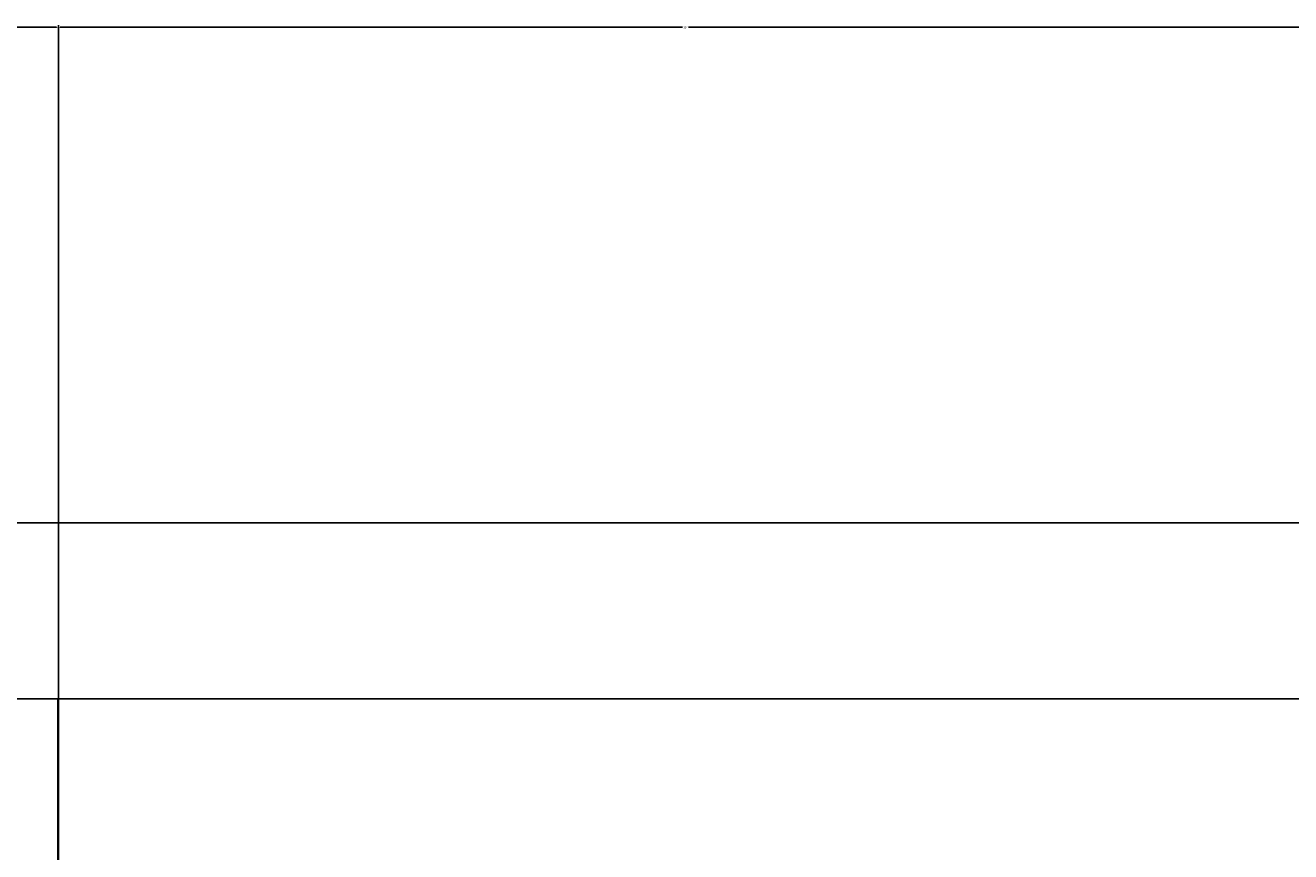
# Model space of a CAD drawing. Units: feet. Extents: x 105 to 1094, y -88 to 588.
# Tile 42 of 59: x 436 to 551, y 513 to 588. Entities that reach past the tile are written whole.
import ezdxf

# ---------------------------------------------------------------- set-up
doc = ezdxf.new("R2010")
doc.units = ezdxf.units.FT
doc.header["$MEASUREMENT"] = 0
for name, color, linetype, lineweight in [('A-ANNO-DIMS', 2, 'Continuous', 18), ('A-FLOR-PROJ', 8, 'Continuous', 25), ('A-WALL', 7, 'Continuous', 35)]:
    doc.layers.add(name, color=color, linetype=linetype, lineweight=lineweight)
doc.styles.get("Standard").update_dxf_attribs({"font": 'arial.ttf'})
doc.dimstyles.get("Standard").update_dxf_attribs({"dimtxt": 0.18, "dimasz": 0.18, "dimexe": 0.18, "dimexo": 0.0625, "dimgap": 0.09, "dimtad": 0, "dimtih": 1, "dimtoh": 1, "dimdec": 4, "dimzin": 0, "dimdsep": 46, "dimtxsty": 'Standard', "dimcen": 0.09, "dimadec": 0, "dimazin": 0, "dimtfac": 1, "dimtdec": 4, "dimtofl": 0, "dimtmove": 0, "dimatfit": 3, "dimfxl": 1, "dimtolj": 1, "dimtzin": 0, "dimarcsym": 0})

# ---------------------------------------------------------------- blocks, each defined once
blk = doc.blocks.new('*D21')
at = {"layer": 'A-ANNO-DIMS', "color": 0, "lineweight": -2, "transparency": 16777216}
for p, q in [((849.63, 543.08), (105.46, 543.08)), ((105.64, 542.9), (105.64, 250.26)), ((105.64, -42.74), (105.64, 249.9)), ((849.63, -42.92), (105.46, -42.92))]:
    blk.add_line(p, q, dxfattribs=at)
at = {"layer": 'A-ANNO-DIMS', "color": 0, "transparency": 16777216}
for points in [[(105.61, 542.9), (105.67, 542.9), (105.64, 543.08)], [(105.61, -42.74), (105.67, -42.74), (105.64, -42.92)]]:
    blk.add_solid(points, dxfattribs=at)
at = {"layer": 'Defpoints', "color": 0, "transparency": 16777216}
for p in [(105.64, 543.08), (849.69, 543.08), (849.69, -42.92)]:
    blk.add_point(p, dxfattribs=at)
at = {"layer": 'A-ANNO-DIMS', "color": 0, "transparency": 16777216, "insert": (105.64, 250.08), "char_height": 0.18, "attachment_point": 5}
blk.add_mtext('\\A1;586', dxfattribs=at)
blk = doc.blocks.new('*D24')
at = {"layer": 'A-ANNO-DIMS', "color": 0, "lineweight": -2, "transparency": 16777216}
for p, q in [((349.69, 543.14), (349.69, 588.31)), ((349.87, 588.13), (393.97, 588.13)), ((438.51, 588.13), (394.41, 588.13)), ((438.69, 527.14), (438.69, 588.31))]:
    blk.add_line(p, q, dxfattribs=at)
at = {"layer": 'A-ANNO-DIMS', "color": 0, "transparency": 16777216}
for points in [[(349.87, 588.16), (349.87, 588.1), (349.69, 588.13)], [(438.51, 588.16), (438.51, 588.1), (438.69, 588.13)]]:
    blk.add_solid(points, dxfattribs=at)
at = {"layer": 'Defpoints', "color": 0, "transparency": 16777216}
for p in [(438.69, 588.13), (349.69, 543.08), (438.69, 527.08)]:
    blk.add_point(p, dxfattribs=at)
at = {"layer": 'A-ANNO-DIMS', "color": 0, "transparency": 16777216, "insert": (394.19, 588.13), "char_height": 0.18, "attachment_point": 5}
blk.add_mtext('\\A1;89', dxfattribs=at)
blk = doc.blocks.new('*D25')
at = {"layer": 'A-ANNO-DIMS', "color": 0, "lineweight": -2, "transparency": 16777216}
for p, q in [((438.69, 527.14), (438.69, 588.31)), ((438.87, 588.13), (495.41, 588.13)), ((552.51, 588.13), (495.97, 588.13)), ((552.69, 471.14), (552.69, 588.31))]:
    blk.add_line(p, q, dxfattribs=at)
at = {"layer": 'A-ANNO-DIMS', "color": 0, "transparency": 16777216}
for points in [[(438.87, 588.16), (438.87, 588.1), (438.69, 588.13)], [(552.51, 588.16), (552.51, 588.1), (552.69, 588.13)]]:
    blk.add_solid(points, dxfattribs=at)
at = {"layer": 'Defpoints', "color": 0, "transparency": 16777216}
for p in [(552.69, 588.13), (438.69, 527.08), (552.69, 471.08)]:
    blk.add_point(p, dxfattribs=at)
at = {"layer": 'A-ANNO-DIMS', "color": 0, "transparency": 16777216, "insert": (495.69, 588.13), "char_height": 0.18, "attachment_point": 5}
blk.add_mtext('\\A1;114', dxfattribs=at)
blk = doc.blocks.new('*D30')
at = {"layer": 'A-ANNO-DIMS', "color": 0, "lineweight": -2, "transparency": 16777216}
for p, q in [((349.75, 543.08), (1093.92, 543.08)), ((1093.74, 542.9), (1093.74, 535.26)), ((1093.74, 527.26), (1093.74, 534.9)), ((349.75, 527.08), (1093.92, 527.08))]:
    blk.add_line(p, q, dxfattribs=at)
at = {"layer": 'A-ANNO-DIMS', "color": 0, "transparency": 16777216}
for points in [[(1093.71, 542.9), (1093.77, 542.9), (1093.74, 543.08)], [(1093.71, 527.26), (1093.77, 527.26), (1093.74, 527.08)]]:
    blk.add_solid(points, dxfattribs=at)
at = {"layer": 'Defpoints', "color": 0, "transparency": 16777216}
for p in [(349.69, 543.08), (349.69, 527.08), (1093.74, 527.08)]:
    blk.add_point(p, dxfattribs=at)
at = {"layer": 'A-ANNO-DIMS', "color": 0, "transparency": 16777216, "insert": (1093.74, 535.08), "char_height": 0.18, "attachment_point": 5}
blk.add_mtext('\\A1;16', dxfattribs=at)
blk = doc.blocks.new('*D31')
at = {"layer": 'A-ANNO-DIMS', "color": 0, "lineweight": -2, "transparency": 16777216}
for p, q in [((438.75, 527.08), (1093.92, 527.08)), ((1093.74, 526.9), (1093.74, 499.26)), ((1093.74, 471.26), (1093.74, 498.9)), ((438.75, 471.08), (1093.92, 471.08))]:
    blk.add_line(p, q, dxfattribs=at)
at = {"layer": 'A-ANNO-DIMS', "color": 0, "transparency": 16777216}
for points in [[(1093.71, 526.9), (1093.77, 526.9), (1093.74, 527.08)], [(1093.71, 471.26), (1093.77, 471.26), (1093.74, 471.08)]]:
    blk.add_solid(points, dxfattribs=at)
at = {"layer": 'Defpoints', "color": 0, "transparency": 16777216}
for p in [(438.69, 527.08), (1093.74, 527.08), (438.69, 471.08)]:
    blk.add_point(p, dxfattribs=at)
at = {"layer": 'A-ANNO-DIMS', "color": 0, "transparency": 16777216, "insert": (1093.74, 499.08), "char_height": 0.18, "attachment_point": 5}
blk.add_mtext('\\A1;56', dxfattribs=at)

msp = doc.modelspace()

# ---------------------------------------------------------------- linework, layer by layer
at = {"layer": 'A-FLOR-PROJ'}
msp.add_line((438.6883, 527.0812), (349.6883, 527.0812), dxfattribs=at)
at = {"layer": 'A-WALL'}
msp.add_line((438.6883, 527.0812), (438.6883, 441.0812), dxfattribs=at)

# ---------------------------------------------------------------- dimensions: what is measured, and where the dimension line sits
at = {"layer": 'A-ANNO-DIMS'}
for base, p1, p2, picture, middle in [((438.6883, 588.1312), (349.6883, 543.0812), (438.6883, 527.0812), '*D24', (394.1883, 588.1312)), ((552.6883, 588.1312), (438.6883, 527.0812), (552.6883, 471.0812), '*D25', (495.6883, 588.1312))]:
    dim = msp.add_linear_dim(base=base, p1=p1, p2=p2, dimstyle='Standard', override={"dimdec": 0, "dimlfac": 1, "dimrnd": 0, "dimzin": 0, "dimdsep": 46, "dimlunit": 2}, dxfattribs=at)
    dim.commit()
    dim.dimension.update_dxf_attribs({"geometry": picture, "text_midpoint": middle})
for base, p1, p2, picture, middle in [((105.6383, 543.0812), (849.6883, -42.9188), (849.6883, 543.0812), '*D21', (105.6383, 250.0812)), ((1093.7383, 527.0812), (349.6883, 543.0812), (349.6883, 527.0812), '*D30', (1093.7383, 535.0812)), ((1093.7383, 527.0812), (438.6883, 471.0812), (438.6883, 527.0812), '*D31', (1093.7383, 499.0812))]:
    dim = msp.add_linear_dim(base=base, p1=p1, p2=p2, angle=90, dimstyle='Standard', override={"dimdec": 0, "dimlfac": 1, "dimrnd": 0, "dimzin": 0, "dimdsep": 46, "dimlunit": 2}, dxfattribs=at)
    dim.commit()
    dim.dimension.update_dxf_attribs({"geometry": picture, "text_midpoint": middle})

doc.saveas('drawing.dxf')
